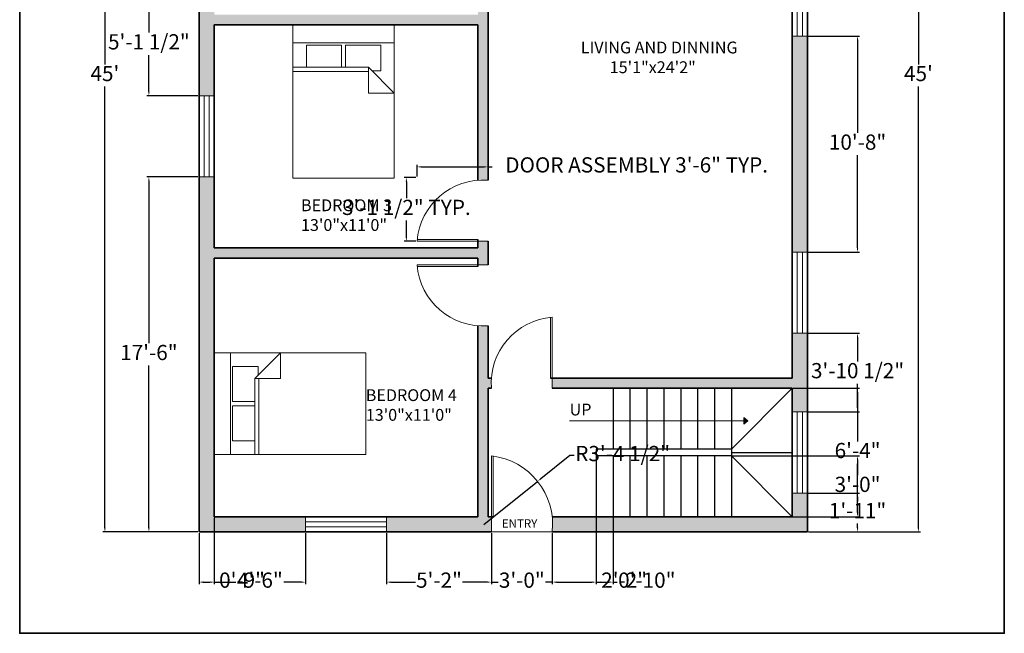
# Model space of a CAD drawing. Units: inches. Extents: x 1994 to 2577, y 1461 to 2158.
# Tile 1 of 2: x 1994 to 2577, y 1461 to 1824. Entities that reach past the tile are written whole.
import ezdxf

# ---------------------------------------------------------------- set-up
doc = ezdxf.new("R2010")
doc.units = ezdxf.units.IN
for name, color, linetype, lineweight in [('A-ANNO-DIMS', 2, 'Continuous', 18), ('A-ANNO-SYMB', 7, 'Continuous', 18), ('A-ANNO-TEXT', 7, 'Continuous', 18), ('A-ANNO-TTLB', 7, 'Continuous', 35), ('A-AREA-IDEN', 7, 'Continuous', 18), ('A-DOOR', 3, 'Continuous', 18), ('A-FLOR-STRS', 7, 'Continuous', 25), ('A-FURN', 9, 'Continuous', 18), ('A-GLAZ', 4, 'Continuous', 18), ('A-WALL', 7, 'Continuous', 35), ('A-WALL-PATT', 8, 'Continuous', 13)]:
    doc.layers.add(name, color=color, linetype=linetype, lineweight=lineweight)
doc.styles.get("Standard").update_dxf_attribs({"font": 'arial.ttf'})
doc.dimstyles.new('ISO-25', dxfattribs={"dimtxt": 9, "dimasz": 2.5, "dimexe": 1.25, "dimexo": 0.625, "dimgap": 2, "dimtad": 0, "dimtih": 1, "dimtoh": 1, "dimdec": 1, "dimlunit": 4, "dimtxsty": 'Standard', "dimcen": 2.5, "dimadec": 0, "dimazin": 0, "dimtfac": 1, "dimtdec": 1, "dimtmove": 0, "dimatfit": 3, "dimfxl": 1, "dimarcsym": 0})

# ---------------------------------------------------------------- blocks, each defined once
blk = doc.blocks.new('Bed - Queen')
for p, q in [((0, -80.00003), (0, 0)), ((0, 0), (59.99999, 0)), ((59.99999, 0), (59.99999, -80.00003)), ((7.99999, -1.2), (28.79998, -1.2)), ((7.99999, -14.4), (7.99999, -1.2)), ((28.79998, -1.2), (28.79998, -14.4)), ((31.19999, -1.2), (51.99999, -1.2)), ((31.19999, -14.4), (31.19999, -1.2)), ((51.99999, -1.2), (51.99999, -16.4)), ((0, -14.4), (44.8, -14.4)), ((44.8, -16.8), (0, -16.8)), ((59.99999, -29.6), (44.8, -14.4)), ((44.8, -14.4), (44.8, -29.6)), ((51.99999, -16.4), (46.79936, -16.4)), ((44.8, -29.6), (59.99999, -29.6)), ((59.99999, -80.00003), (0, -80.00003))]:
    blk.add_line(p, q)
blk = doc.blocks.new('*D4')
at = {"layer": 'A-ANNO-DIMS', "color": 0, "lineweight": -2, "transparency": 16777216}
for p, q in [((2461.02, 2061.02), (2527.29, 2061.02)), ((2526.04, 2058.52), (2526.04, 1797.59)), ((2526.04, 1523.52), (2526.04, 1784.44)), ((2461.02, 1521.02), (2527.29, 1521.02))]:
    blk.add_line(p, q, dxfattribs=at)
at = {"layer": 'A-ANNO-DIMS', "color": 0, "transparency": 16777216}
for points in [[(2525.63, 2058.52), (2526.46, 2058.52), (2526.04, 2061.02)], [(2525.63, 1523.52), (2526.46, 1523.52), (2526.04, 1521.02)]]:
    blk.add_solid(points, dxfattribs=at)
at = {"layer": 'Defpoints', "color": 0, "transparency": 16777216}
for p in [(2460.39, 2061.02), (2460.39, 1521.02), (2526.04, 1521.02)]:
    blk.add_point(p, dxfattribs=at)
at = {"layer": 'A-ANNO-DIMS', "color": 0, "transparency": 16777216, "insert": (2526.04, 1791.02), "char_height": 9, "attachment_point": 5}
blk.add_mtext("45'", dxfattribs=at)
blk = doc.blocks.new('*D8')
at = {"layer": 'A-ANNO-DIMS', "color": 0, "lineweight": -2, "transparency": 16777216}
for p, q in [((2099.77, 2061.02), (2043.44, 2061.02)), ((2044.69, 2058.52), (2044.69, 1797.59)), ((2044.69, 1523.52), (2044.69, 1784.44)), ((2099.77, 1521.02), (2043.44, 1521.02))]:
    blk.add_line(p, q, dxfattribs=at)
at = {"layer": 'A-ANNO-DIMS', "color": 0, "transparency": 16777216}
for points in [[(2044.27, 2058.52), (2045.11, 2058.52), (2044.69, 2061.02)], [(2044.27, 1523.52), (2045.11, 1523.52), (2044.69, 1521.02)]]:
    blk.add_solid(points, dxfattribs=at)
at = {"layer": 'Defpoints', "color": 0, "transparency": 16777216}
for p in [(2100.39, 2061.02), (2044.69, 1521.02), (2100.39, 1521.02)]:
    blk.add_point(p, dxfattribs=at)
at = {"layer": 'A-ANNO-DIMS', "color": 0, "transparency": 16777216, "insert": (2044.69, 1791.02), "char_height": 9, "attachment_point": 5}
blk.add_mtext("45'", dxfattribs=at)
blk = doc.blocks.new('WIN-48IN')
for p, q in [((9, 48), (0, 48)), ((0, 48), (0, 0)), ((3, 48), (3, 0)), ((6, 48), (6, 0)), ((9, 0), (0, 0))]:
    blk.add_line(p, q)
blk = doc.blocks.new('DOOR-SWING-36IN')
for p, q in [((36, 1), (0, 1)), ((36, 0), (0, 0)), ((36, 0), (42, 0))]:
    blk.add_line(p, q)
blk.add_arc((39, -3), 39.12, 85.60129, 175.60129)
blk = doc.blocks.new('*D13')
at = {"layer": 'A-ANNO-DIMS', "color": 0, "lineweight": -2, "transparency": 16777216}
for p, q in [((2229.39, 1731.3), (2229.39, 1738.22)), ((2231.89, 1736.97), (2268.89, 1736.97)), ((2271.39, 1731.3), (2271.39, 1738.22)), ((2271.39, 1736.97), (2273.89, 1736.97))]:
    blk.add_line(p, q, dxfattribs=at)
at = {"layer": 'A-ANNO-DIMS', "color": 0, "transparency": 16777216}
for points in [[(2231.89, 1737.39), (2231.89, 1736.56), (2229.39, 1736.97)], [(2268.89, 1737.39), (2268.89, 1736.56), (2271.39, 1736.97)]]:
    blk.add_solid(points, dxfattribs=at)
at = {"layer": 'Defpoints', "color": 0, "transparency": 16777216}
for p in [(2271.39, 1736.97), (2229.39, 1730.67), (2271.39, 1730.67)]:
    blk.add_point(p, dxfattribs=at)
at = {"layer": 'A-ANNO-DIMS', "color": 0, "transparency": 16777216, "insert": (2359.34, 1736.97), "char_height": 9, "attachment_point": 5}
blk.add_mtext('DOOR ASSEMBLY 3\'-6" TYP.', dxfattribs=at)
blk = doc.blocks.new('*D14')
at = {"layer": 'A-ANNO-DIMS', "color": 0, "lineweight": -2, "transparency": 16777216}
for p, q in [((2228.77, 1730.67), (2221.84, 1730.67)), ((2223.09, 1728.17), (2223.09, 1718.5)), ((2223.09, 1695.52), (2223.09, 1705.19)), ((2228.77, 1693.02), (2221.84, 1693.02))]:
    blk.add_line(p, q, dxfattribs=at)
at = {"layer": 'A-ANNO-DIMS', "color": 0, "transparency": 16777216}
for points in [[(2222.67, 1728.17), (2223.51, 1728.17), (2223.09, 1730.67)], [(2222.67, 1695.52), (2223.51, 1695.52), (2223.09, 1693.02)]]:
    blk.add_solid(points, dxfattribs=at)
at = {"layer": 'Defpoints', "color": 0, "transparency": 16777216}
for p in [(2223.09, 1730.67), (2229.39, 1730.67), (2229.39, 1693.02)]:
    blk.add_point(p, dxfattribs=at)
at = {"layer": 'A-ANNO-DIMS', "color": 0, "transparency": 16777216, "insert": (2223.09, 1711.84), "char_height": 9, "attachment_point": 5}
blk.add_mtext('3\'-1 1/2" TYP.', dxfattribs=at)
blk = doc.blocks.new('*D21')
at = {"layer": 'A-ANNO-DIMS', "color": 0, "lineweight": -2, "transparency": 16777216}
for p, q in [((2109.39, 1529.39), (2109.39, 1490.12)), ((2100.39, 1520.39), (2100.39, 1490.12)), ((2102.89, 1491.37), (2106.89, 1491.37)), ((2109.39, 1491.37), (2111.89, 1491.37))]:
    blk.add_line(p, q, dxfattribs=at)
at = {"layer": 'A-ANNO-DIMS', "color": 0, "transparency": 16777216}
for points in [[(2102.89, 1491.78), (2102.89, 1490.95), (2100.39, 1491.37)], [(2106.89, 1491.78), (2106.89, 1490.95), (2109.39, 1491.37)]]:
    blk.add_solid(points, dxfattribs=at)
at = {"layer": 'Defpoints', "color": 0, "transparency": 16777216}
for p in [(2109.39, 1530.02), (2100.39, 1521.02), (2109.39, 1491.37)]:
    blk.add_point(p, dxfattribs=at)
at = {"layer": 'A-ANNO-DIMS', "color": 0, "transparency": 16777216, "insert": (2125.85, 1491.37), "char_height": 9, "attachment_point": 5}
blk.add_mtext('0\'-9"', dxfattribs=at)
blk = doc.blocks.new('*D23')
at = {"layer": 'A-ANNO-DIMS', "color": 0, "lineweight": -2, "transparency": 16777216}
for p, q in [((2109.39, 1529.39), (2109.39, 1490.12)), ((2163.39, 1520.39), (2163.39, 1490.12)), ((2111.89, 1491.37), (2122.25, 1491.37)), ((2160.89, 1491.37), (2150.53, 1491.37))]:
    blk.add_line(p, q, dxfattribs=at)
at = {"layer": 'A-ANNO-DIMS', "color": 0, "transparency": 16777216}
for points in [[(2111.89, 1491.78), (2111.89, 1490.95), (2109.39, 1491.37)], [(2160.89, 1491.78), (2160.89, 1490.95), (2163.39, 1491.37)]]:
    blk.add_solid(points, dxfattribs=at)
at = {"layer": 'Defpoints', "color": 0, "transparency": 16777216}
for p in [(2109.39, 1530.02), (2163.39, 1521.02), (2163.39, 1491.37)]:
    blk.add_point(p, dxfattribs=at)
at = {"layer": 'A-ANNO-DIMS', "color": 0, "transparency": 16777216, "insert": (2136.39, 1491.37), "char_height": 9, "attachment_point": 5}
blk.add_mtext('4\'-6"', dxfattribs=at)
blk = doc.blocks.new('*D24')
at = {"layer": 'A-ANNO-DIMS', "color": 0, "lineweight": -2, "transparency": 16777216}
for p, q in [((2211.39, 1520.39), (2211.39, 1490.12)), ((2273.39, 1520.39), (2273.39, 1490.12)), ((2213.89, 1491.37), (2228.43, 1491.37)), ((2270.89, 1491.37), (2256.35, 1491.37))]:
    blk.add_line(p, q, dxfattribs=at)
at = {"layer": 'A-ANNO-DIMS', "color": 0, "transparency": 16777216}
for points in [[(2213.89, 1491.78), (2213.89, 1490.95), (2211.39, 1491.37)], [(2270.89, 1491.78), (2270.89, 1490.95), (2273.39, 1491.37)]]:
    blk.add_solid(points, dxfattribs=at)
at = {"layer": 'Defpoints', "color": 0, "transparency": 16777216}
for p in [(2211.39, 1521.02), (2273.39, 1521.02), (2273.39, 1491.37)]:
    blk.add_point(p, dxfattribs=at)
at = {"layer": 'A-ANNO-DIMS', "color": 0, "transparency": 16777216, "insert": (2242.39, 1491.37), "char_height": 9, "attachment_point": 5}
blk.add_mtext('5\'-2"', dxfattribs=at)
blk = doc.blocks.new('*D25')
at = {"layer": 'A-ANNO-DIMS', "color": 0, "lineweight": -2, "transparency": 16777216}
for p, q in [((2273.39, 1520.39), (2273.39, 1490.12)), ((2309.39, 1520.39), (2309.39, 1490.12)), ((2270.89, 1491.37), (2268.39, 1491.37)), ((2273.39, 1491.37), (2277.43, 1491.37)), ((2309.39, 1491.37), (2305.35, 1491.37)), ((2311.89, 1491.37), (2314.39, 1491.37))]:
    blk.add_line(p, q, dxfattribs=at)
at = {"layer": 'A-ANNO-DIMS', "color": 0, "transparency": 16777216}
for points in [[(2270.89, 1491.78), (2270.89, 1490.95), (2273.39, 1491.37)], [(2311.89, 1491.78), (2311.89, 1490.95), (2309.39, 1491.37)]]:
    blk.add_solid(points, dxfattribs=at)
at = {"layer": 'Defpoints', "color": 0, "transparency": 16777216}
for p in [(2273.39, 1521.02), (2309.39, 1521.02), (2309.39, 1491.37)]:
    blk.add_point(p, dxfattribs=at)
at = {"layer": 'A-ANNO-DIMS', "color": 0, "transparency": 16777216, "insert": (2291.39, 1491.37), "char_height": 9, "attachment_point": 5}
blk.add_mtext('3\'-0"', dxfattribs=at)
blk = doc.blocks.new('*D26')
at = {"layer": 'A-ANNO-DIMS', "color": 0, "lineweight": -2, "transparency": 16777216}
for p, q in [((2461.02, 1544.02), (2491.29, 1544.02)), ((2490.04, 1541.52), (2490.04, 1539.03)), ((2461.02, 1521.02), (2491.29, 1521.02)), ((2490.04, 1523.52), (2490.04, 1526))]:
    blk.add_line(p, q, dxfattribs=at)
at = {"layer": 'A-ANNO-DIMS', "color": 0, "transparency": 16777216}
for points in [[(2489.62, 1541.52), (2490.46, 1541.52), (2490.04, 1544.02)], [(2489.62, 1523.52), (2490.46, 1523.52), (2490.04, 1521.02)]]:
    blk.add_solid(points, dxfattribs=at)
at = {"layer": 'Defpoints', "color": 0, "transparency": 16777216}
for p in [(2460.39, 1544.02), (2490.04, 1544.02), (2460.39, 1521.02)]:
    blk.add_point(p, dxfattribs=at)
at = {"layer": 'A-ANNO-DIMS', "color": 0, "transparency": 16777216, "insert": (2490.04, 1532.52), "char_height": 9, "attachment_point": 5}
blk.add_mtext('1\'-11"', dxfattribs=at)
blk = doc.blocks.new('*D27')
at = {"layer": 'A-ANNO-DIMS', "color": 0, "lineweight": -2, "transparency": 16777216}
for p, q in [((2461.02, 1638.53), (2491.29, 1638.53)), ((2490.04, 1636.03), (2490.04, 1621.93)), ((2490.04, 1594.52), (2490.04, 1608.62)), ((2461.02, 1592.02), (2491.29, 1592.02))]:
    blk.add_line(p, q, dxfattribs=at)
at = {"layer": 'A-ANNO-DIMS', "color": 0, "transparency": 16777216}
for points in [[(2489.62, 1636.03), (2490.46, 1636.03), (2490.04, 1638.53)], [(2489.62, 1594.52), (2490.46, 1594.52), (2490.04, 1592.02)]]:
    blk.add_solid(points, dxfattribs=at)
at = {"layer": 'Defpoints', "color": 0, "transparency": 16777216}
for p in [(2460.39, 1638.53), (2490.04, 1638.53), (2460.39, 1592.02)]:
    blk.add_point(p, dxfattribs=at)
at = {"layer": 'A-ANNO-DIMS', "color": 0, "transparency": 16777216, "insert": (2490.04, 1615.27), "char_height": 9, "attachment_point": 5}
blk.add_mtext('3\'-10 1/2"', dxfattribs=at)
blk = doc.blocks.new('*D28')
at = {"layer": 'A-ANNO-DIMS', "color": 0, "lineweight": -2, "transparency": 16777216}
for p, q in [((2461.02, 1814.34), (2491.29, 1814.34)), ((2490.04, 1811.84), (2490.04, 1757.03)), ((2490.04, 1689.03), (2490.04, 1743.84)), ((2461.02, 1686.53), (2491.29, 1686.53))]:
    blk.add_line(p, q, dxfattribs=at)
at = {"layer": 'A-ANNO-DIMS', "color": 0, "transparency": 16777216}
for points in [[(2489.62, 1811.84), (2490.46, 1811.84), (2490.04, 1814.34)], [(2489.62, 1689.03), (2490.46, 1689.03), (2490.04, 1686.53)]]:
    blk.add_solid(points, dxfattribs=at)
at = {"layer": 'Defpoints', "color": 0, "transparency": 16777216}
for p in [(2460.39, 1814.34), (2490.04, 1814.34), (2460.39, 1686.53)]:
    blk.add_point(p, dxfattribs=at)
at = {"layer": 'A-ANNO-DIMS', "color": 0, "transparency": 16777216, "insert": (2490.04, 1750.44), "char_height": 9, "attachment_point": 5}
blk.add_mtext('10\'-8"', dxfattribs=at)
blk = doc.blocks.new('*D30')
at = {"layer": 'A-ANNO-DIMS', "color": 0, "lineweight": -2, "transparency": 16777216}
for p, q in [((2099.77, 1731.02), (2069.49, 1731.02)), ((2070.74, 1728.52), (2070.74, 1632.61)), ((2070.74, 1523.52), (2070.74, 1619.42)), ((2099.77, 1521.02), (2069.49, 1521.02))]:
    blk.add_line(p, q, dxfattribs=at)
at = {"layer": 'A-ANNO-DIMS', "color": 0, "transparency": 16777216}
for points in [[(2070.32, 1728.52), (2071.16, 1728.52), (2070.74, 1731.02)], [(2070.32, 1523.52), (2071.16, 1523.52), (2070.74, 1521.02)]]:
    blk.add_solid(points, dxfattribs=at)
at = {"layer": 'Defpoints', "color": 0, "transparency": 16777216}
for p in [(2070.74, 1731.02), (2100.39, 1731.02), (2100.39, 1521.02)]:
    blk.add_point(p, dxfattribs=at)
at = {"layer": 'A-ANNO-DIMS', "color": 0, "transparency": 16777216, "insert": (2070.74, 1626.02), "char_height": 9, "attachment_point": 5}
blk.add_mtext('17\'-6"', dxfattribs=at)
blk = doc.blocks.new('*D31')
at = {"layer": 'A-ANNO-DIMS', "color": 0, "lineweight": -2, "transparency": 16777216}
for p, q in [((2099.77, 1840.52), (2069.49, 1840.52)), ((2070.74, 1838.02), (2070.74, 1816.42)), ((2070.74, 1781.52), (2070.74, 1803.11)), ((2099.77, 1779.02), (2069.49, 1779.02))]:
    blk.add_line(p, q, dxfattribs=at)
at = {"layer": 'A-ANNO-DIMS', "color": 0, "transparency": 16777216}
for points in [[(2070.32, 1838.02), (2071.16, 1838.02), (2070.74, 1840.52)], [(2070.32, 1781.52), (2071.16, 1781.52), (2070.74, 1779.02)]]:
    blk.add_solid(points, dxfattribs=at)
at = {"layer": 'Defpoints', "color": 0, "transparency": 16777216}
for p in [(2070.74, 1840.52), (2100.39, 1840.52), (2100.39, 1779.02)]:
    blk.add_point(p, dxfattribs=at)
at = {"layer": 'A-ANNO-DIMS', "color": 0, "transparency": 16777216, "insert": (2070.74, 1809.77), "char_height": 9, "attachment_point": 5}
blk.add_mtext('5\'-1 1/2"', dxfattribs=at)
blk = doc.blocks.new('*D35')
at = {"layer": 'A-ANNO-DIMS', "color": 0, "lineweight": -2, "transparency": 16777216}
for p, q in [((2416.02, 1566.02), (2491.29, 1566.02)), ((2490.04, 1563.52), (2490.04, 1554.61)), ((2490.04, 1532.52), (2490.04, 1541.42)), ((2416.02, 1530.02), (2491.29, 1530.02))]:
    blk.add_line(p, q, dxfattribs=at)
at = {"layer": 'A-ANNO-DIMS', "color": 0, "transparency": 16777216}
for points in [[(2489.62, 1563.52), (2490.46, 1563.52), (2490.04, 1566.02)], [(2489.62, 1532.52), (2490.46, 1532.52), (2490.04, 1530.02)]]:
    blk.add_solid(points, dxfattribs=at)
at = {"layer": 'Defpoints', "color": 0, "transparency": 16777216}
for p in [(2415.39, 1566.02), (2490.04, 1566.02), (2415.39, 1530.02)]:
    blk.add_point(p, dxfattribs=at)
at = {"layer": 'A-ANNO-DIMS', "color": 0, "transparency": 16777216, "insert": (2490.04, 1548.02), "char_height": 9, "attachment_point": 5}
blk.add_mtext('3\'-0"', dxfattribs=at)
blk = doc.blocks.new('*D36')
at = {"layer": 'A-ANNO-DIMS', "color": 0, "lineweight": -2, "transparency": 16777216}
for p, q in [((2335.39, 1529.39), (2335.39, 1490.12)), ((2345.39, 1529.39), (2345.39, 1490.12)), ((2337.89, 1491.37), (2342.89, 1491.37)), ((2345.39, 1491.37), (2347.89, 1491.37))]:
    blk.add_line(p, q, dxfattribs=at)
at = {"layer": 'A-ANNO-DIMS', "color": 0, "transparency": 16777216}
for points in [[(2337.89, 1491.78), (2337.89, 1490.95), (2335.39, 1491.37)], [(2342.89, 1491.78), (2342.89, 1490.95), (2345.39, 1491.37)]]:
    blk.add_solid(points, dxfattribs=at)
at = {"layer": 'Defpoints', "color": 0, "transparency": 16777216}
for p in [(2335.39, 1530.02), (2345.39, 1530.02), (2345.39, 1491.37)]:
    blk.add_point(p, dxfattribs=at)
at = {"layer": 'A-ANNO-DIMS', "color": 0, "transparency": 16777216, "insert": (2365.35, 1491.37), "char_height": 9, "attachment_point": 5}
blk.add_mtext('0\'-10"', dxfattribs=at)
blk = doc.blocks.new('*D37')
at = {"layer": 'A-ANNO-DIMS', "color": 0, "lineweight": -2, "transparency": 16777216}
for p, q in [((2335.39, 1529.39), (2335.39, 1490.12)), ((2309.39, 1520.39), (2309.39, 1490.12)), ((2311.89, 1491.37), (2332.89, 1491.37)), ((2335.39, 1491.37), (2337.89, 1491.37))]:
    blk.add_line(p, q, dxfattribs=at)
at = {"layer": 'A-ANNO-DIMS', "color": 0, "transparency": 16777216}
for points in [[(2311.89, 1491.78), (2311.89, 1490.95), (2309.39, 1491.37)], [(2332.89, 1491.78), (2332.89, 1490.95), (2335.39, 1491.37)]]:
    blk.add_solid(points, dxfattribs=at)
at = {"layer": 'Defpoints', "color": 0, "transparency": 16777216}
for p in [(2335.39, 1530.02), (2309.39, 1521.02), (2335.39, 1491.37)]:
    blk.add_point(p, dxfattribs=at)
at = {"layer": 'A-ANNO-DIMS', "color": 0, "transparency": 16777216, "insert": (2351.93, 1491.37), "char_height": 9, "attachment_point": 5}
blk.add_mtext('2\'-2"', dxfattribs=at)
blk = doc.blocks.new('*D38')
at = {"layer": 'A-ANNO-DIMS', "color": 0, "lineweight": -2, "transparency": 16777216}
for p, q in [((2452.02, 1606.02), (2491.29, 1606.02)), ((2490.04, 1603.52), (2490.04, 1574.61)), ((2490.04, 1532.52), (2490.04, 1561.42)), ((2452.02, 1530.02), (2491.29, 1530.02))]:
    blk.add_line(p, q, dxfattribs=at)
at = {"layer": 'A-ANNO-DIMS', "color": 0, "transparency": 16777216}
for points in [[(2489.62, 1603.52), (2490.46, 1603.52), (2490.04, 1606.02)], [(2489.62, 1532.52), (2490.46, 1532.52), (2490.04, 1530.02)]]:
    blk.add_solid(points, dxfattribs=at)
at = {"layer": 'Defpoints', "color": 0, "transparency": 16777216}
for p in [(2451.39, 1606.02), (2490.04, 1606.02), (2451.39, 1530.02)]:
    blk.add_point(p, dxfattribs=at)
at = {"layer": 'A-ANNO-DIMS', "color": 0, "transparency": 16777216, "insert": (2490.04, 1568.02), "char_height": 9, "attachment_point": 5}
blk.add_mtext('6\'-4"', dxfattribs=at)
blk = doc.blocks.new('*D39')
at = {"layer": 'A-ANNO-DIMS', "color": 0, "lineweight": -2, "transparency": 16777216}
for p, q in [((2319.8, 1566.25), (2302.66, 1552.53)), ((2322.3, 1566.25), (2319.8, 1566.25)), ((2268.89, 1525.52), (2300.71, 1550.97))]:
    blk.add_line(p, q, dxfattribs=at)
at = {"layer": 'A-ANNO-DIMS', "color": 0, "transparency": 16777216}
blk.add_solid([(2302.4, 1552.86), (2302.92, 1552.21), (2300.71, 1550.97)], dxfattribs=at)
at = {"layer": 'Defpoints', "color": 0, "transparency": 16777216}
for p in [(2300.71, 1550.97), (2268.89, 1525.52)]:
    blk.add_point(p, dxfattribs=at)
at = {"layer": 'A-ANNO-DIMS', "color": 0, "transparency": 16777216, "insert": (2351.06, 1566.25), "char_height": 9, "attachment_point": 5}
blk.add_mtext('R3\'-4 1/2"', dxfattribs=at)

msp = doc.modelspace()

# ---------------------------------------------------------------- hatches: boundary and pattern name
at = {"layer": 'A-ANNO-SYMB'}
h = msp.add_hatch(color=256, dxfattribs=at)
h.dxf.hatch_style = 1
h.paths.add_polyline_path([(2422.79, 1588.76), (2422.82, 1586.75), (2425.21, 1586.75)])
h.paths.add_polyline_path([(2425.21, 1586.75), (2422.82, 1586.75), (2422.85, 1584.79)])
at = {"layer": 'A-WALL-PATT'}
h = msp.add_hatch(color=256, dxfattribs=at)
h.dxf.hatch_style = 1
h.paths.add_polyline_path([(2287.39, 2061.02), (2100.39, 2061.02), (2100.39, 2004.02), (2109.39, 2004.02), (2109.39, 2052.02), (2265.39, 2052.02), (2265.39, 1946.02, -0.038405), (2271.39, 1946.02), (2271.39, 1950.02), (2273.39, 1950.02), (2273.39, 1956.02), (2271.39, 1956.02), (2271.39, 2052.02), (2287.39, 2052.02)])
h.paths.add_polyline_path([(2460.39, 2061.02), (2311.39, 2061.02), (2311.39, 2052.02), (2327.39, 2052.02), (2327.39, 1956.02), (2297.39, 1956.02, -0.055385), (2297.39, 1950.02), (2327.39, 1950.02), (2327.39, 1946.02, -0.038405), (2333.39, 1946.02), (2333.39, 2052.02), (2451.39, 2052.02), (2451.39, 2004.02), (2460.39, 2004.02)])
h.paths.add_polyline_path([(2460.39, 1956.02), (2451.39, 1956.02), (2451.39, 1908.02), (2333.39, 1908.02), (2333.39, 1910.02), (2327.39, 1910.02), (2327.39, 1902.02), (2451.39, 1902.02), (2451.39, 1862.34), (2460.39, 1862.34)])
h.paths.add_polyline_path([(2109.39, 1956.02), (2100.39, 1956.02), (2100.39, 1888.52), (2109.39, 1888.52), (2109.39, 1902.02), (2265.39, 1902.02), (2265.39, 1866.02), (2271.39, 1866.02), (2271.39, 1910.02), (2265.39, 1910.02), (2265.39, 1908.02), (2109.39, 1908.02)])
h.paths.add_polyline_path([(2460.39, 1814.34), (2451.39, 1814.34), (2451.39, 1686.53), (2460.39, 1686.53)])
h.paths.add_polyline_path([(2271.39, 1830.02), (2265.39, 1830.02), (2265.39, 1827.02), (2109.39, 1827.02), (2109.39, 1840.52), (2100.39, 1840.52), (2100.39, 1779.02), (2109.39, 1779.02), (2109.39, 1821.02), (2265.39, 1821.02), (2265.39, 1729.02, -0.038405), (2271.39, 1729.02)])
h.paths.add_polyline_path([(2109.39, 1683.02), (2265.39, 1683.02), (2265.39, 1679.02), (2271.39, 1679.02), (2271.39, 1693.02), (2265.39, 1693.02), (2265.39, 1689.02), (2109.39, 1689.02), (2109.39, 1731.02), (2100.39, 1731.02), (2100.39, 1521.02), (2163.39, 1521.02), (2163.39, 1530.02), (2109.39, 1530.02)])
h.paths.add_polyline_path([(2273.39, 1530.02), (2271.39, 1530.02), (2271.39, 1606.02), (2273.39, 1606.02, -0.038405), (2273.39, 1612.02), (2271.39, 1612.02), (2271.39, 1643.02, -0.038405), (2265.39, 1643.02), (2265.39, 1530.02), (2211.39, 1530.02), (2211.39, 1521.02), (2273.39, 1521.02)])
h.paths.add_polyline_path([(2460.39, 1544.02), (2451.39, 1544.02), (2451.39, 1530.02), (2309.39, 1530.02, -0.055385), (2309.39, 1521.02), (2460.39, 1521.02)])
h.paths.add_polyline_path([(2460.39, 1638.53), (2451.39, 1638.53), (2451.39, 1612.02), (2309.39, 1612.02), (2309.39, 1606.02), (2451.39, 1606.02), (2451.39, 1592.02), (2460.39, 1592.02)])

# ---------------------------------------------------------------- linework, layer by layer
at = {"layer": 'A-ANNO-SYMB'}
for p, q in [((2319.66, 1586.75), (2425.21, 1586.75)), ((2425.21, 1586.75), (2422.79, 1588.76)), ((2422.79, 1588.76), (2422.85, 1584.79)), ((2422.85, 1584.79), (2425.21, 1586.75))]:
    msp.add_line(p, q, dxfattribs=at)
at = {"layer": 'A-ANNO-TTLB'}
msp.add_lwpolyline([(1994.29, 2157.92), (2576.88, 2157.92), (2576.88, 1461.09), (1994.29, 1461.09)], close=True, dxfattribs=at)
at = {"layer": 'A-DOOR'}
for p, q in [((2273.39, 1530.02), (2273.39, 1566.02)), ((2274.39, 1530.02), (2274.39, 1566.02)), ((2273.39, 1530.02), (2273.39, 1521.02)), ((2273.39, 1521.02), (2309.39, 1521.02))]:
    msp.add_line(p, q, dxfattribs=at)
msp.add_arc((2268.89, 1525.52), 40.75, 353.65981, 83.65981, dxfattribs=at)
at = {"layer": 'A-FLOR-STRS'}
for p, q in [((2345.39, 1606.02), (2345.39, 1570.02)), ((2355.39, 1606.02), (2355.39, 1570.02)), ((2365.39, 1606.02), (2365.39, 1570.02)), ((2375.39, 1606.02), (2375.39, 1570.02)), ((2385.39, 1606.02), (2385.39, 1570.02)), ((2395.39, 1606.02), (2395.39, 1570.02)), ((2405.39, 1606.02), (2405.39, 1570.02)), ((2415.39, 1606.02), (2415.39, 1530.02)), ((2415.39, 1570.02), (2451.39, 1606.02)), ((2415.39, 1570.02), (2335.39, 1570.02)), ((2335.39, 1570.02), (2335.39, 1530.02)), ((2415.39, 1570.02), (2415.39, 1566.02)), ((2415.39, 1568.02), (2451.39, 1568.02)), ((2415.39, 1566.02), (2335.39, 1566.02)), ((2345.39, 1566.02), (2345.39, 1530.02)), ((2355.39, 1566.02), (2355.39, 1530.02)), ((2365.39, 1566.02), (2365.39, 1530.02)), ((2375.39, 1566.02), (2375.39, 1530.02)), ((2385.39, 1566.02), (2385.39, 1530.02)), ((2395.39, 1566.02), (2395.39, 1530.02)), ((2405.39, 1566.02), (2405.39, 1530.02)), ((2415.39, 1566.02), (2451.39, 1530.02))]:
    msp.add_line(p, q, dxfattribs=at)
at = {"layer": 'A-FURN'}
for p, q in [((2155.92, 1810.25), (2155.92, 1821.02)), ((2215.92, 1810.25), (2215.92, 1821.02)), ((2119.07, 1626.91), (2109.39, 1626.91)), ((2119.07, 1566.91), (2109.39, 1566.91))]:
    msp.add_line(p, q, dxfattribs=at)
at = {"layer": 'A-WALL'}
for p, q in [((2100.39, 1521.02), (2100.39, 2061.02)), ((2460.39, 2061.02), (2460.39, 1521.02)), ((2451.39, 1902.02), (2451.39, 1612.02)), ((2271.39, 1729.02), (2271.39, 1830.02)), ((2109.39, 1821.02), (2265.39, 1821.02)), ((2109.39, 1689.02), (2109.39, 1821.02)), ((2265.39, 1729.02), (2265.39, 1821.02)), ((2265.39, 1689.02), (2265.39, 1694.02)), ((2271.39, 1679.02), (2271.39, 1693.02)), ((2109.39, 1689.02), (2265.39, 1689.02)), ((2109.39, 1530.02), (2109.39, 1683.02)), ((2109.39, 1683.02), (2265.39, 1683.02)), ((2265.39, 1678.02), (2265.39, 1683.02)), ((2265.39, 1530.02), (2265.39, 1643.02)), ((2271.39, 1612.02), (2271.39, 1643.02)), ((2273.39, 1612.02), (2271.39, 1612.02)), ((2451.39, 1612.02), (2308.39, 1612.02)), ((2271.39, 1530.02), (2271.39, 1606.02)), ((2273.39, 1606.02), (2271.39, 1606.02)), ((2451.39, 1606.02), (2309.39, 1606.02)), ((2451.39, 1606.02), (2451.39, 1530.02)), ((2451.39, 1606.02), (2451.39, 1530.02)), ((2265.39, 1530.02), (2109.39, 1530.02)), ((2274.39, 1530.02), (2271.39, 1530.02)), ((2451.39, 1530.02), (2309.39, 1530.02)), ((2273.39, 1521.02), (2100.39, 1521.02)), ((2460.39, 1521.02), (2309.39, 1521.02))]:
    msp.add_line(p, q, dxfattribs=at)

# ---------------------------------------------------------------- block references
at = {"layer": 'A-DOOR'}
msp.add_blockref('DOOR-SWING-36IN', (2229.39, 1693.02), dxfattribs=at)
at = {"layer": 'A-DOOR', "extrusion": (0, 0, -1), "zscale": -1}
for p, rotation in [((-2229.39, 1679.02), 180), ((-2309.39, 1648.02), 269.9999999999968)]:
    msp.add_blockref('DOOR-SWING-36IN', p, dxfattribs=dict(at, rotation=rotation))
at = {"layer": 'A-FURN'}
msp.add_blockref('Bed - Queen', (2155.92, 1810.25), dxfattribs=at)
at = {"layer": 'A-FURN', "rotation": 90}
msp.add_blockref('Bed - Queen', (2119.07, 1566.91), dxfattribs=at)
at = {"layer": 'A-GLAZ'}
for p in [(2451.39, 1814.34), (2100.39, 1731.02), (2451.39, 1638.53), (2451.39, 1544.02)]:
    msp.add_blockref('WIN-48IN', p, dxfattribs=at)
at = {"layer": 'A-GLAZ', "rotation": 89.99999999999604}
msp.add_blockref('WIN-48IN', (2211.39, 1521.02), dxfattribs=at)

# ---------------------------------------------------------------- texts
at = {"layer": 'A-ANNO-TEXT', "attachment_point": 1}
for s, width, insert, char_height in [('UP', 2.863, (2319.66, 1596.94), 7), ('ENTRY', 28.0925, (2279.58, 1528.54), 5)]:
    msp.add_mtext_dynamic_manual_height_columns(s, width=width, gutter_width=12.5, heights=[0], dxfattribs=dict(at, insert=insert, char_height=char_height))
at = {"layer": 'A-AREA-IDEN', "char_height": 7, "attachment_point": 1}
for s, width, insert in [('{\\fArial|b1|i0|c0|p34;LIVING AND DINNING\\P        15\'1"x24\'2"}', 109.8059, (2326.29, 1811.07)), ('{\\fArial|b1|i0|c0|p34;BEDROOM 3\\P13\'0"x11\'0"}', 98.1837, (2160.73, 1717.75)), ('{\\fArial|b1|i0|c0|p34;BEDROOM 4\\P13\'0"x11\'0"}', 66.3224, (2199.07, 1605.45))]:
    msp.add_mtext_dynamic_manual_height_columns(s, width=width, gutter_width=12.5, heights=[0], dxfattribs=dict(at, insert=insert))

# ---------------------------------------------------------------- dimensions: what is measured, and where the dimension line sits
at = {"layer": 'A-ANNO-DIMS'}
for base, p1, p2, override, picture, middle in [((2044.69, 1521.02), (2100.39, 2061.02), (2100.39, 1521.02), {"dimclrd": 0, "dimclre": 0, "dimclrt": 0}, '*D8', (2044.69, 1791.02)), ((2526.04, 1521.02), (2460.39, 2061.02), (2460.39, 1521.02), {"dimclrd": 0, "dimclre": 0, "dimclrt": 0}, '*D4', (2526.04, 1791.02)), ((2070.74, 1840.52), (2100.39, 1779.02), (2100.39, 1840.52), {"dimdec": 1, "dimlfac": 1, "dimrnd": 0, "dimzin": 1, "dimdsep": 46, "dimlunit": 4, "dimfrac": 2}, '*D31', (2070.74, 1809.77)), ((2490.04, 1814.34), (2460.39, 1686.53), (2460.39, 1814.34), {"dimdec": 1, "dimlfac": 1, "dimrnd": 0, "dimzin": 1, "dimdsep": 46, "dimlunit": 4, "dimfrac": 2}, '*D28', (2490.04, 1750.44)), ((2070.74, 1731.02), (2100.39, 1521.02), (2100.39, 1731.02), {"dimdec": 1, "dimlfac": 1, "dimrnd": 0, "dimzin": 1, "dimdsep": 46, "dimlunit": 4, "dimfrac": 2}, '*D30', (2070.74, 1626.02)), ((2490.04, 1638.53), (2460.39, 1592.02), (2460.39, 1638.53), {"dimdec": 1, "dimlfac": 1, "dimrnd": 0, "dimzin": 1, "dimdsep": 46, "dimlunit": 4, "dimfrac": 2}, '*D27', (2490.04, 1615.27)), ((2490.04, 1606.02), (2451.39, 1530.02), (2451.39, 1606.02), {"dimdec": 1, "dimlfac": 1, "dimrnd": 0, "dimzin": 1, "dimdsep": 46, "dimlunit": 4, "dimfrac": 2}, '*D38', (2490.04, 1568.02)), ((2490.04, 1566.02), (2415.39, 1530.02), (2415.39, 1566.02), {"dimdec": 1, "dimlfac": 1, "dimrnd": 0, "dimzin": 1, "dimdsep": 46, "dimlunit": 4, "dimfrac": 2}, '*D35', (2490.04, 1548.02)), ((2490.04, 1544.02), (2460.39, 1521.02), (2460.39, 1544.02), {"dimdec": 1, "dimlfac": 1, "dimrnd": 0, "dimzin": 1, "dimdsep": 46, "dimlunit": 4, "dimfrac": 2}, '*D26', (2490.04, 1532.52))]:
    dim = msp.add_linear_dim(base=base, p1=p1, p2=p2, angle=90, dimstyle='ISO-25', override=override, dxfattribs=at)
    dim.commit()
    dim.dimension.update_dxf_attribs({"geometry": picture, "text_midpoint": middle})
dim = msp.add_linear_dim(base=(2271.39, 1736.97), p1=(2229.39, 1730.67), p2=(2271.39, 1730.67), text='DOOR ASSEMBLY <> TYP.', dimstyle='ISO-25', override={"dimdec": 1, "dimlfac": 1, "dimrnd": 0, "dimzin": 1, "dimdsep": 46, "dimlunit": 4, "dimfrac": 2}, dxfattribs=at)
dim.commit()
dim.dimension.update_dxf_attribs({"geometry": '*D13', "text_midpoint": (2359.34, 1736.97)})
dim = msp.add_linear_dim(base=(2223.0901, 1730.6734), p1=(2229.3901, 1693.0166), p2=(2229.3901, 1730.6734), angle=90, text='<> TYP.', dimstyle='ISO-25', override={"dimdec": 1, "dimlfac": 1, "dimrnd": 0, "dimzin": 1, "dimdsep": 46, "dimlunit": 4, "dimfrac": 2}, dxfattribs=at)
dim.commit()
dim.dimension.update_dxf_attribs({"geometry": '*D14', "text_midpoint": (2223.0901, 1711.845)})
dim = msp.add_radius_dim(center=(2268.89, 1525.52), mpoint=(2300.71, 1550.97), dimstyle='ISO-25', override={"dimdec": 1, "dimlfac": 1, "dimrnd": 0, "dimzin": 1, "dimdsep": 46, "dimlunit": 4, "dimfrac": 2}, dxfattribs=at)
dim.commit()
dim.dimension.update_dxf_attribs({"geometry": '*D39', "text_midpoint": (2351.06, 1566.25), "dimtype": 164})
for base, p1, p2, picture, middle in [((2109.39, 1491.37), (2100.39, 1521.02), (2109.39, 1530.02), '*D21', (2125.85, 1491.37)), ((2163.39, 1491.37), (2109.39, 1530.02), (2163.39, 1521.02), '*D23', (2136.39, 1491.37)), ((2335.39, 1491.37), (2309.39, 1521.02), (2335.39, 1530.02), '*D37', (2351.93, 1491.37)), ((2345.39, 1491.37), (2335.39, 1530.02), (2345.39, 1530.02), '*D36', (2365.35, 1491.37)), ((2273.39, 1491.37), (2211.39, 1521.02), (2273.39, 1521.02), '*D24', (2242.39, 1491.37)), ((2309.39, 1491.37), (2273.39, 1521.02), (2309.39, 1521.02), '*D25', (2291.39, 1491.37))]:
    dim = msp.add_linear_dim(base=base, p1=p1, p2=p2, dimstyle='ISO-25', override={"dimdec": 1, "dimlfac": 1, "dimrnd": 0, "dimzin": 1, "dimdsep": 46, "dimlunit": 4, "dimfrac": 2}, dxfattribs=at)
    dim.commit()
    dim.dimension.update_dxf_attribs({"geometry": picture, "text_midpoint": middle})

doc.saveas('drawing.dxf')
